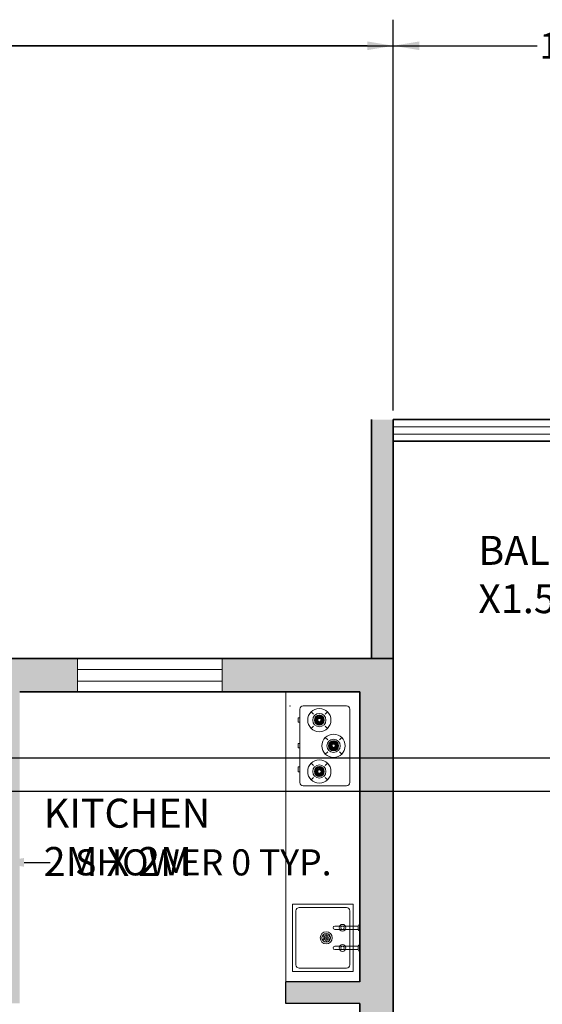
# Model space of a CAD drawing. Units: metres. Extents: x 2031 to 2061.8, y 1886.4 to 1909.8.
# Tile 6 of 10: x 2042.3 to 2045.9, y 1903 to 1909.8. Entities that reach past the tile are written whole.
import ezdxf

# ---------------------------------------------------------------- set-up
doc = ezdxf.new("R2010")
doc.units = ezdxf.units.M
for name, color, linetype, lineweight in [('A-ANNO-DIMS', 2, 'Continuous', 18), ('A-AREA-IDEN', 7, 'Continuous', 18), ('A-EQPM', 8, 'Continuous', 18), ('A-FLOR-CASE', 8, 'Continuous', 18), ('A-FLOR-FIXT', 8, 'Continuous', 18), ('A-WALL-PATT', 252, 'Continuous', 13), ('furniture', 24, 'Continuous', 13), ('grills', 5, 'Continuous', 13), ('inner walls', 4, 'Continuous', 25), ('windows', 30, 'Continuous', 18)]:
    doc.layers.add(name, color=color, linetype=linetype, lineweight=lineweight)
doc.layers.add('outer walls', color=1, linetype='Continuous', lineweight=35, plot=False)
doc.styles.get("Standard").update_dxf_attribs({"font": 'arial.ttf'})
doc.dimstyles.get("Standard").update_dxf_attribs({"dimtxt": 0.18, "dimasz": 0.18, "dimexe": 0.18, "dimexo": 0.0625, "dimgap": 0.09, "dimtad": 0, "dimtih": 1, "dimtoh": 1, "dimdec": 4, "dimzin": 0, "dimdsep": 46, "dimtxsty": 'Standard', "dimcen": 0.09, "dimadec": 0, "dimazin": 0, "dimtfac": 1, "dimtdec": 4, "dimtofl": 0, "dimtmove": 0, "dimatfit": 3, "dimfxl": 1, "dimtolj": 1, "dimtzin": 0, "dimarcsym": 0})

# ---------------------------------------------------------------- blocks, each defined once
blk = doc.blocks.new('sink')
for p, q in [((0, 0), (-22.00000000000001, 0)), ((0, 0), (0, 0)), ((-20.00000000000023, -2.999999999999995), (-2.000000000000178, -3)), ((-19.99999999999959, -22.99999999999988), (-20.00000000000023, -2.999999999999995)), ((-18.99999999999966, -20.99999999999994), (-19.00000000000017, -4.999999999999996)), ((-18.00000000000017, -3.999999999999996), (-4.000000000000113, -3.999999999999999)), ((-3.000000000000114, -5), (-2.999999999999607, -20.99999999999988)), ((-2.000000000000178, -3), (-1.999999999999543, -22.99999999999988)), ((-0.5000000000000026, -9.499999999999813), (-7.500000000000004, -9.499999999999812)), ((-0.5000000000000028, -10.49999999999981), (-7.500000000000004, -10.49999999999981)), ((-0.5000000000000026, -9.499999999999813), (-0.5000000000000028, -10.49999999999981)), ((-2.4e-15, -8.999999999999813), (-2.9e-15, -10.99999999999981)), ((-0.500000000000004, -15.49999999999981), (-7.500000000000005, -15.49999999999981)), ((-0.5000000000000044, -16.49999999999981), (-7.500000000000005, -16.49999999999981)), ((-0.500000000000004, -15.49999999999981), (-0.5000000000000044, -16.49999999999981)), ((-3.9e-15, -14.99999999999981), (-4.4e-15, -16.99999999999981)), ((-19.99999999999959, -22.99999999999988), (-1.999999999999543, -22.99999999999988)), ((-17.99999999999966, -21.99999999999988), (-3.999999999999607, -21.99999999999989))]:
    blk.add_line(p, q)
for centre, radius in [((-10.00000000000014, -12.99999999999968), 1.794435724606955), ((-5.180961460384426, -9.999999999999812), 1), ((-5.180961460384426, -9.999999999999812), 0.5), ((-10.00000000000014, -12.99999999999968), 1.294435724606955), ((-10.66093109696162, -12.61841125325318), 0.25), ((-10.66093109696162, -13.38158874674618), 0.25), ((-10.00000000000014, -12.23682250650668), 0.25), ((-10.00000000000014, -12.99999999999968), 0.25), ((-10.00000000000014, -13.76317749349269), 0.25), ((-9.33906890303867, -12.61841125325318), 0.25), ((-9.33906890303867, -13.38158874674618), 0.25), ((-5.180961460384427, -15.99999999999981), 1), ((-5.180961460384427, -15.99999999999981), 0.5)]:
    blk.add_circle(centre, radius)
for centre, radius, start, end in [((-18.00000000000017, -4.999999999999996), 1, 89.99999999999999, 180), ((-4.000000000000115, -5), 1, 0, 89.99999999999999), ((-7.500000000000004, -9.999999999999812), 0.5, 89.99999999999999, 270), ((0.010449978117122, -9.510449978116938), 0.5105569333604445, 91.17280055555744, 178.8271994444424), ((0.0104499781171218, -10.48955002188269), 0.5105569333604445, 181.1728005555574, 268.8271994444423), ((-7.500000000000005, -15.99999999999981), 0.5, 89.99999999999999, 270), ((0.0104499781171206, -15.51044997811693), 0.5105569333604445, 91.17280055555744, 178.8271994444424), ((0.0104499781171203, -16.48955002188269), 0.5105569333604445, 181.1728005555573, 268.8271994444423), ((-17.99999999999966, -20.99999999999988), 1, 180, 270), ((-3.999999999999607, -20.99999999999988), 1, 270, 0)]:
    blk.add_arc(centre, radius, start, end)
blk = doc.blocks.new('stove')
at = {"layer": 'furniture'}
h = blk.add_hatch(dxfattribs=at)
h.set_pattern_fill('HEX', color=256, angle=180, style=0)
h.set_pattern_definition([(360, (23.99999999999982, 24.99999999999816), (1e-16, 0.216506351), [0.125, -0.25]), (119.9999999999999, (23.99999999999982, 24.99999999999816), (-0.1875000000466704, -0.1082531754999999), [0.1249999999999998, -0.2499999999999996]), (59.99999999999994, (24.12499999999982, 24.99999999999816), (-0.1875000000466704, 0.1082531755000001), [0.125, -0.25])])
h.paths.add_polyline_path([(10.36428182591571, 19.71316705046143, 1), (7.364281825915714, 19.71316705046143, 1)])
h.paths.add_polyline_path([(9.364281825915715, 19.71316705046143, -1), (8.364281825915715, 19.71316705046143, -1)], flags=16)
h = blk.add_hatch(dxfattribs=at)
h.set_pattern_fill('HEX', color=256, angle=180, style=0)
h.set_pattern_definition([(180, (-2.000000000000001, 6.713167050462818), (-1e-16, -0.216506351), [0.125, -0.25]), (300, (-2.000000000000001, 6.713167050462818), (0.1875000000466704, 0.1082531754999999), [0.1249999999999999, -0.2499999999999998]), (239.9999999999999, (-2.125000000000001, 6.713167050462818), (0.1875000000466704, -0.1082531755000001), [0.125, -0.25])])
h.paths.add_polyline_path([(14.6357181740841, 11.99999999999954, 1), (11.6357181740841, 11.99999999999954, 1)])
h.paths.add_polyline_path([(12.6357181740841, 11.99999999999954, -1), (13.6357181740841, 11.99999999999954, -1)], flags=16)
h = blk.add_hatch(dxfattribs=at)
h.set_pattern_fill('HEX', color=256, angle=180, style=0)
h.set_pattern_definition([(360, (23.99999999999982, -0.9999999999999342), (-1e-16, -0.216506351), [0.125, -0.25]), (239.9999999999999, (23.99999999999982, -0.9999999999999342), (-0.1875000000466704, 0.1082531755), [0.1249999999999999, -0.2499999999999998]), (300, (24.12499999999982, -0.9999999999999342), (-0.1875000000466704, -0.1082531755), [0.125, -0.2499999999999999])])
h.paths.add_polyline_path([(10.36428182591571, 4.2868329495368, 1), (7.364281825915714, 4.2868329495368, 1)])
h.paths.add_polyline_path([(9.364281825915715, 4.2868329495368, -1), (8.364281825915715, 4.2868329495368, -1)], flags=16)
for p, q in [((4.000000000000007, 23.99999999999909), (17, 23.99999999999908)), ((3, 1.000000000000003), (3.000000000000007, 22.99999999999909)), ((6.389408091762671, 22.18804078461422), (7.09651487294905, 21.48093400342751)), ((10.6320487788818, 21.48093400342809), (11.33915556006851, 22.18804078461447)), ((18, 22.99999999999908), (18, 0.9999999999991327)), ((3.000000000000007, 19.86017834974973), (2.500000000000003, 19.86017834974973)), ((2.500000000000003, 19.86017834974973), (2.500000000000003, 18.36017834974973)), ((2.500000000000003, 18.36017834974973), (3.000000000000003, 18.36017834974973)), ((6.389408091762675, 17.23829331630864), (7.096514872949061, 17.94540009749535)), ((10.63204877888179, 17.94540009749477), (11.3391555600685, 17.23829331630838)), ((2.500000000000003, 12.64999999999954), (2.500000000000003, 11.34999999999955)), ((3.000000000000003, 12.64999999999954), (2.500000000000003, 12.64999999999954)), ((11.36795122111803, 13.7677669529662), (10.66084443993131, 14.47487373415259)), ((15.61059190823715, 14.47487373415233), (14.90348512705075, 13.76776695296562)), ((2.500000000000003, 11.34999999999955), (3.000000000000003, 11.34999999999955)), ((11.36795122111803, 10.23223304703288), (10.66084443993131, 9.525126265846504)), ((15.61059190823714, 9.525126265846753), (14.90348512705077, 10.23223304703346)), ((6.389408091762671, 6.761706683689592), (7.096514872949061, 6.054599902502877)), ((10.63204877888178, 6.05459990250346), (11.3391555600685, 6.761706683689842)), ((2.500000000000003, 4.936832949536799), (2.500000000000003, 3.636832949536802)), ((3.000000000000003, 4.936832949536799), (2.500000000000003, 4.936832949536799)), ((2.500000000000003, 3.636832949536802), (3.000000000000003, 3.636832949536802)), ((16.99999999999994, -8.669e-13), (3.999999999999946, 3.6e-15)), ((6.389408091762668, 1.811959215384014), (7.096514872949043, 2.519065996570723)), ((10.63204877888179, 2.519065996570138), (11.3391555600685, 1.81195921538376))]:
    blk.add_line(p, q, dxfattribs=at)
for centre, radius in [((8.864281825915715, 19.71316705046143), 3.499999999999999), ((8.864281825915715, 19.71316705046143), 1.999999999999999), ((8.864281825915715, 19.71316705046143), 1.5), ((8.864281825915715, 19.71316705046143), 0.5000000000000004), ((13.1357181740841, 11.99999999999954), 3.499999999999999), ((13.1357181740841, 11.99999999999954), 1.999999999999999), ((13.1357181740841, 11.99999999999954), 1.5), ((13.1357181740841, 11.99999999999954), 0.5000000000000004), ((8.864281825915715, 4.286832949536801), 3.499999999999999), ((8.864281825915715, 4.2868329495368), 1.999999999999999), ((8.864281825915715, 4.2868329495368), 1.5), ((8.864281825915715, 4.2868329495368), 0.5000000000000004)]:
    blk.add_circle(centre, radius, dxfattribs=at)
for centre, start, end in [((4.000000000000007, 22.99999999999909), 90, 180), ((17, 22.99999999999908), 0, 90), ((4, 1.000000000000003), 180, 269.9999999999968), ((17, 0.9999999999991331), 269.9999999999968, 0)]:
    blk.add_arc(centre, 1, start, end, dxfattribs=at)
at = {"layer": 'furniture', "ltscale": 9}
blk.add_point((0, 0), dxfattribs=at)
blk = doc.blocks.new('WIN-1000')
for p, q in [((2.274e-13, 0), (0, 0.2299999999997908)), ((1.000000000000227, 9.095e-13), (1, 0.2300000000007003)), ((2.274e-13, 0.1549999999997453), (1.000000000000227, 0.1549999999997453)), ((2.274e-13, 0.0749999999998181), (1.000000000000227, 0.0749999999998181))]:
    blk.add_line(p, q)
blk = doc.blocks.new('BALCONY-GUARD-2500')
for p, q in [((4.547e-13, 0.0500000000010914), (2.5, 0.0500000000006367)), ((4.547e-13, 6.821e-13), (2.5, 4.547e-13))]:
    blk.add_line(p, q)
blk = doc.blocks.new('*D32')
at = {"layer": 'A-ANNO-DIMS', "color": 0, "lineweight": -2, "transparency": 16777216}
for p, q in [((2041.621106728857, 1904.024726820454), (2041.441106728857, 1904.024726820454)), ((2041.801106728857, 1904.009143718862), (2041.801106728857, 1903.844726820454)), ((2042.113886051581, 1904.009143718862), (2042.113886051581, 1903.844726820454)), ((2042.293886051581, 1904.024726820454), (2042.473886051581, 1904.024726820454))]:
    blk.add_line(p, q, dxfattribs=at)
at = {"layer": 'A-ANNO-DIMS', "color": 0, "transparency": 16777216}
for points in [[(2041.621106728857, 1904.054726820454), (2041.621106728857, 1903.994726820454), (2041.801106728857, 1904.024726820454)], [(2042.293886051581, 1904.054726820454), (2042.293886051581, 1903.994726820454), (2042.113886051581, 1904.024726820454)]]:
    blk.add_solid(points, dxfattribs=at)
at = {"layer": 'Defpoints', "color": 0, "transparency": 16777216}
for p in [(2041.801106728857, 1904.071643718862), (2042.113886051581, 1904.071643718862), (2042.113886051581, 1904.024726820454)]:
    blk.add_point(p, dxfattribs=at)
at = {"layer": 'A-ANNO-DIMS', "color": 0, "transparency": 16777216, "insert": (2043.532337620476, 1904.024726820454), "char_height": 0.18, "attachment_point": 5}
blk.add_mtext('\\A1;SHOWER 0 TYP.', dxfattribs=at)
blk = doc.blocks.new('*D47')
at = {"layer": 'A-ANNO-DIMS', "color": 0, "lineweight": -2, "transparency": 16777216}
for p, q in [((2037.813886, 1906.456584), (2037.813886, 1909.84065)), ((2044.843886, 1907.143703), (2044.843886, 1909.84065)), ((2037.993886, 1909.66065), (2041.005843708049, 1909.66065)), ((2044.663886, 1909.66065), (2041.651928291951, 1909.66065))]:
    blk.add_line(p, q, dxfattribs=at)
at = {"layer": 'A-ANNO-DIMS', "color": 0, "transparency": 16777216}
for points in [[(2037.993886, 1909.69065), (2037.993886, 1909.63065), (2037.813886, 1909.66065)], [(2044.663886, 1909.69065), (2044.663886, 1909.63065), (2044.843886, 1909.66065)]]:
    blk.add_solid(points, dxfattribs=at)
at = {"layer": 'Defpoints', "color": 0, "transparency": 16777216}
for p in [(2044.843886, 1909.66065), (2044.843886, 1907.081203), (2037.813886, 1906.394084)]:
    blk.add_point(p, dxfattribs=at)
at = {"layer": 'A-ANNO-DIMS', "color": 0, "transparency": 16777216, "insert": (2041.328886, 1909.66065), "char_height": 0.18, "attachment_point": 5}
blk.add_mtext('\\A1;7.03', dxfattribs=at)
blk = doc.blocks.new('*D48')
at = {"layer": 'A-ANNO-DIMS', "color": 0, "lineweight": -2, "transparency": 16777216}
for p, q in [((2044.843886, 1907.143703), (2044.843886, 1909.84065)), ((2047.343886, 1907.143703), (2047.343886, 1909.84065)), ((2045.023886, 1909.66065), (2045.837821879946, 1909.66065)), ((2047.163886, 1909.66065), (2046.349950120055, 1909.66065))]:
    blk.add_line(p, q, dxfattribs=at)
at = {"layer": 'A-ANNO-DIMS', "color": 0, "transparency": 16777216}
for points in [[(2045.023886, 1909.69065), (2045.023886, 1909.63065), (2044.843886, 1909.66065)], [(2047.163886, 1909.69065), (2047.163886, 1909.63065), (2047.343886, 1909.66065)]]:
    blk.add_solid(points, dxfattribs=at)
at = {"layer": 'Defpoints', "color": 0, "transparency": 16777216}
for p in [(2047.343886, 1909.66065), (2044.843886, 1907.081203), (2047.343886, 1907.081203)]:
    blk.add_point(p, dxfattribs=at)
at = {"layer": 'A-ANNO-DIMS', "color": 0, "transparency": 16777216, "insert": (2046.093886, 1909.66065), "char_height": 0.18, "attachment_point": 5}
blk.add_mtext('\\A1;2.5', dxfattribs=at)
blk = doc.blocks.new('*D58')
at = {"layer": 'A-ANNO-DIMS', "color": 0, "lineweight": -2, "transparency": 16777216}
for p, q in [((2040.415705, 1896.633713), (2040.415705, 1909.84065)), ((2052.040038, 1896.633713), (2052.040038, 1909.84065)), ((2040.595705, 1909.66065), (2045.773082959755, 1909.66065)), ((2051.860038, 1909.66065), (2046.682660040246, 1909.66065))]:
    blk.add_line(p, q, dxfattribs=at)
at = {"layer": 'A-ANNO-DIMS', "color": 0, "transparency": 16777216}
for points in [[(2040.595705, 1909.69065), (2040.595705, 1909.63065), (2040.415705, 1909.66065)], [(2051.860038, 1909.69065), (2051.860038, 1909.63065), (2052.040038, 1909.66065)]]:
    blk.add_solid(points, dxfattribs=at)
at = {"layer": 'Defpoints', "color": 0, "transparency": 16777216}
for p in [(2052.040038, 1909.66065), (2040.415705, 1896.571213), (2052.040038, 1896.571213)]:
    blk.add_point(p, dxfattribs=at)
at = {"layer": 'A-ANNO-DIMS', "color": 0, "transparency": 16777216, "insert": (2046.227871500001, 1909.66065), "char_height": 0.18, "attachment_point": 5}
blk.add_mtext('\\A1;11.624', dxfattribs=at)
blk = doc.blocks.new('*D60')
at = {"layer": 'A-ANNO-DIMS', "color": 0, "lineweight": -2, "transparency": 16777216}
for p, q in [((2031.744780000002, 1904.924084000001), (2031.744780000002, 1905.104084000001)), ((2056.161386000001, 1904.744084), (2031.564780000002, 1904.744084)), ((2055.931386000001, 1904.514084000001), (2031.564780000002, 1904.514084000001)), ((2031.744780000002, 1904.334084000001), (2031.744780000002, 1904.154084000001)), ((2031.744780000002, 1904.154084000001), (2031.564780000002, 1904.154084000001))]:
    blk.add_line(p, q, dxfattribs=at)
at = {"layer": 'A-ANNO-DIMS', "color": 0, "transparency": 16777216}
for points in [[(2031.714780000002, 1904.924084000001), (2031.774780000002, 1904.924084000001), (2031.744780000002, 1904.744084)], [(2031.714780000002, 1904.334084000001), (2031.774780000002, 1904.334084000001), (2031.744780000002, 1904.514084000001)]]:
    blk.add_solid(points, dxfattribs=at)
at = {"layer": 'Defpoints', "color": 0, "transparency": 16777216}
for p in [(2056.223886000001, 1904.744084), (2031.744780000002, 1904.514084000001), (2055.993886000001, 1904.514084000001)]:
    blk.add_point(p, dxfattribs=at)
at = {"layer": 'A-ANNO-DIMS', "color": 0, "transparency": 16777216, "insert": (2031.241001009552, 1904.154084), "char_height": 0.18, "attachment_point": 5}
blk.add_mtext('\\A1;0.23', dxfattribs=at)

msp = doc.modelspace()

# ---------------------------------------------------------------- hatches: boundary and pattern name
at = {"layer": 'A-WALL-PATT'}
h = msp.add_hatch(color=256, dxfattribs=at)
h.dxf.hatch_style = 1
h.paths.add_polyline_path([(2044.843886051581, 1905.431202972395), (2043.662726773602, 1905.431202972395), (2043.662726773602, 1905.201202972395), (2044.613886051581, 1905.201202972395), (2044.613886051581, 1903.201202972395), (2044.10203621828, 1903.201202972395), (2044.10203621828, 1903.051247813867), (2044.613886051581, 1903.051202972395), (2044.613784550147, 1901.892599367488), (2044.843481671829, 1901.892599367488)])
h.paths.add_polyline_path([(2044.843886051581, 1907.081202972395), (2044.693886051581, 1907.081202972395), (2044.693886051581, 1905.431202972395), (2044.843886051581, 1905.431202972395)])
h.paths.add_polyline_path([(2042.662726773602, 1905.431202972395), (2041.608725591668, 1905.431202972395), (2041.608725591668, 1905.201202972395), (2042.113886051581, 1905.201202972395), (2042.113886051581, 1903.201202972395), (2042.11388605158, 1903.200960518025), (2041.878665859902, 1903.200960518025, -0.0160568248018428), (2041.87111792116, 1903.201202972395), (2040.613886051581, 1903.201202972395), (2040.463886051581, 1903.201202972395), (2040.46388605158, 1903.051202972395), (2042.263886051581, 1903.051202972395), (2042.263886051581, 1905.201202972395), (2042.662726773602, 1905.201202972395)])
h.paths.add_polyline_path([(2040.804457664849, 1903.878793012381), (2041.776183449296, 1903.878793012381), (2041.776183449296, 1904.438513339803), (2040.804457664849, 1904.438513339803)], flags=25)
h.paths.add_polyline_path([(2042.05521314868, 1900.945611707966), (2043.754121743495, 1900.945611707966), (2043.754121743495, 1901.691905477861), (2042.05521314868, 1901.691905477861)], flags=9)
h.paths.add_polyline_path([(2038.540886554753, 1905.248744193212), (2040.159440442883, 1905.248744193212), (2040.159440442883, 1905.995037963107), (2038.540886554753, 1905.995037963107)], flags=9)
h.paths.add_polyline_path([(2038.693906317999, 1902.140700941841), (2040.392814912815, 1902.140700941841), (2040.392814912815, 1902.886994711737), (2038.693906317999, 1902.886994711737)], flags=9)
h.paths.add_polyline_path([(2042.359230799286, 1903.821641126969), (2043.685560949354, 1903.821641126969), (2043.685560949354, 1904.567934896864), (2042.359230799286, 1904.567934896864)], flags=9)

# ---------------------------------------------------------------- linework, layer by layer
at = {"layer": 'A-FLOR-CASE', "ltscale": 0.3}
msp.add_line((2044.10203621828, 1905.201445426765), (2044.10203621828, 1903.201202972395), dxfattribs=at)
at = {"layer": 'inner walls'}
for p, q in [((2044.613886051581, 1903.201202972395), (2044.10203621828, 1903.201202972395)), ((2044.10203621828, 1903.051247813867), (2044.10203621828, 1903.201202972395)), ((2044.613886051581, 1903.051202972395), (2044.10203621828, 1903.051247813867))]:
    msp.add_line(p, q, dxfattribs=at)
at = {"layer": 'outer walls'}
for p, q in [((2044.693886051581, 1905.431202972395), (2044.693886051581, 1907.081202972395)), ((2044.843886051581, 1905.431202972395), (2044.843886051581, 1907.081202972395)), ((2044.843886051581, 1907.081202972395), (2047.493886051581, 1907.081202972395)), ((2044.843886051581, 1906.931202972395), (2047.343886051581, 1906.931202972395)), ((2040.613886051581, 1905.431202972395), (2044.843886051581, 1905.431202972395)), ((2044.843886051581, 1905.431202972395), (2044.843193535108, 1899.371202985826)), ((2042.263886051582, 1905.201202972395), (2044.613886051581, 1905.201202972395)), ((2044.613886051581, 1905.201202972395), (2044.613886051581, 1903.201202972395)), ((2044.613886051581, 1903.051202972395), (2044.61356365894, 1899.371202985826))]:
    msp.add_line(p, q, dxfattribs=at)

# ---------------------------------------------------------------- block references
at = {"layer": 'A-EQPM', "xscale": -0.0229818441149355, "yscale": 0.0229818441149355, "zscale": 0.0229818441149355, "rotation": 180}
msp.add_blockref('stove', (2044.129660727241, 1905.104951542376), dxfattribs=at)
at = {"layer": 'A-FLOR-FIXT', "xscale": -0.0232659015136525, "yscale": 0.0232659015136525, "zscale": 0.0232659015136525, "rotation": 180}
msp.add_blockref('sink', (2044.613886051581, 1903.201202972395), dxfattribs=at)
at = {"layer": 'grills'}
msp.add_blockref('BALCONY-GUARD-2500', (2044.843886051581, 1906.981202972394), dxfattribs=at)
at = {"layer": 'windows'}
msp.add_blockref('WIN-1000', (2042.662726773602, 1905.201202972395), dxfattribs=at)

# ---------------------------------------------------------------- texts
at = {"layer": 'A-AREA-IDEN', "char_height": 0.2, "attachment_point": 7}
for s, width, insert in [('BALCONY        2.5M X1.5M', 2.302330104705106, (2045.430973233493, 1905.744656013613)), ('KITCHEN \\P2M X 2M', 1.594746697714981, (2042.429694646489, 1903.930713432562))]:
    msp.add_mtext_dynamic_manual_height_columns(s, width=width, gutter_width=12.5, heights=[0], dxfattribs=dict(at, insert=insert))

# ---------------------------------------------------------------- dimensions: what is measured, and where the dimension line sits
at = {"layer": 'A-ANNO-DIMS'}
for base, p1, p2, override, picture, middle in [((2044.843886, 1909.66065), (2037.813886, 1906.394084), (2044.843886, 1907.081203), {"dimdec": 2, "dimlfac": 1, "dimrnd": 0, "dimzin": 0, "dimdsep": 46, "dimlunit": 2}, '*D47', (2041.328886, 1909.66065)), ((2052.040038, 1909.66065), (2040.415705, 1896.571213), (2052.040038, 1896.571213), {"dimdec": 3, "dimlfac": 1, "dimrnd": 0, "dimzin": 0, "dimdsep": 46, "dimlunit": 2}, '*D58', (2046.227871500001, 1909.66065)), ((2047.343886, 1909.66065), (2044.843886, 1907.081203), (2047.343886, 1907.081203), {"dimdec": 1, "dimlfac": 1, "dimrnd": 0, "dimzin": 0, "dimdsep": 46, "dimlunit": 2}, '*D48', (2046.093886, 1909.66065))]:
    dim = msp.add_linear_dim(base=base, p1=p1, p2=p2, dimstyle='Standard', override=override, dxfattribs=at)
    dim.commit()
    dim.dimension.update_dxf_attribs({"geometry": picture, "text_midpoint": middle})
dim = msp.add_linear_dim(base=(2031.744780000002, 1904.514084000001), p1=(2056.223886000001, 1904.744084), p2=(2055.993886, 1904.514084), angle=90, dimstyle='Standard', override={"dimdec": 2, "dimlfac": 1, "dimrnd": 0, "dimzin": 0, "dimdsep": 46, "dimlunit": 2}, dxfattribs=at)
dim.commit()
dim.dimension.update_dxf_attribs({"geometry": '*D60', "text_midpoint": (2031.241001009552, 1904.154084)})
dim = msp.add_linear_dim(base=(2042.113886051581, 1904.024726820454), p1=(2041.801106728857, 1904.071643718862), p2=(2042.113886051581, 1904.071643718862), text='SHOWER <> TYP.', dimstyle='Standard', override={"dimdec": 0, "dimlfac": 1, "dimrnd": 0, "dimzin": 0, "dimdsep": 46, "dimlunit": 2}, dxfattribs=at)
dim.commit()
dim.dimension.update_dxf_attribs({"geometry": '*D32', "text_midpoint": (2043.532337620476, 1904.024726820454)})

doc.saveas('drawing.dxf')
